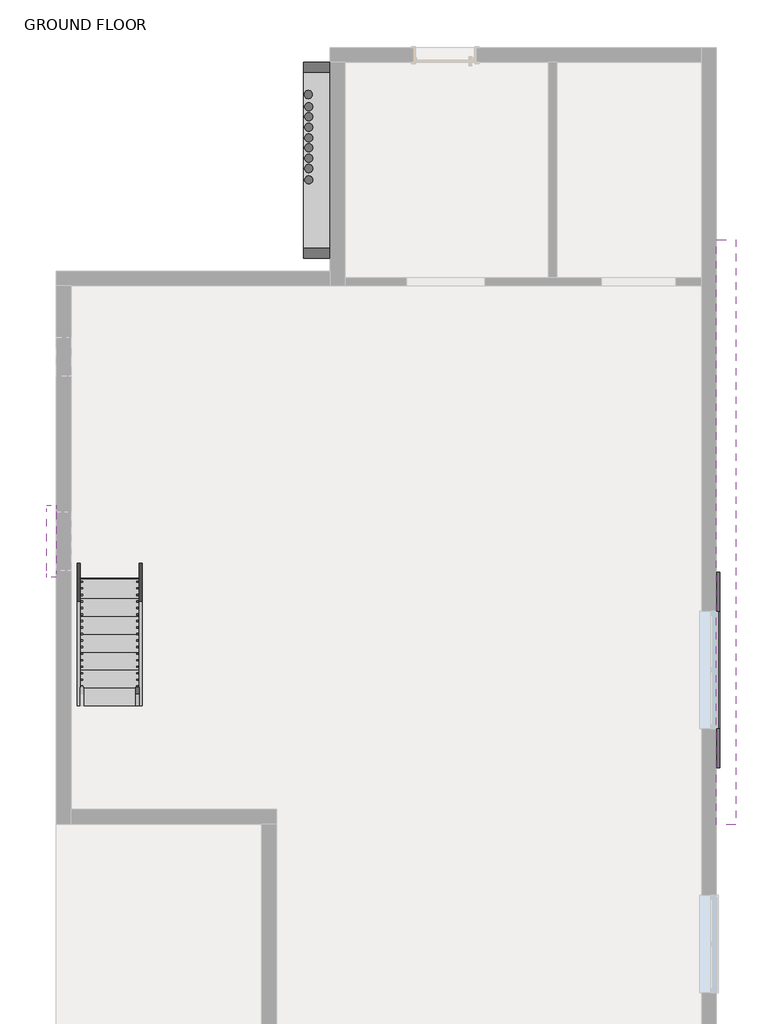
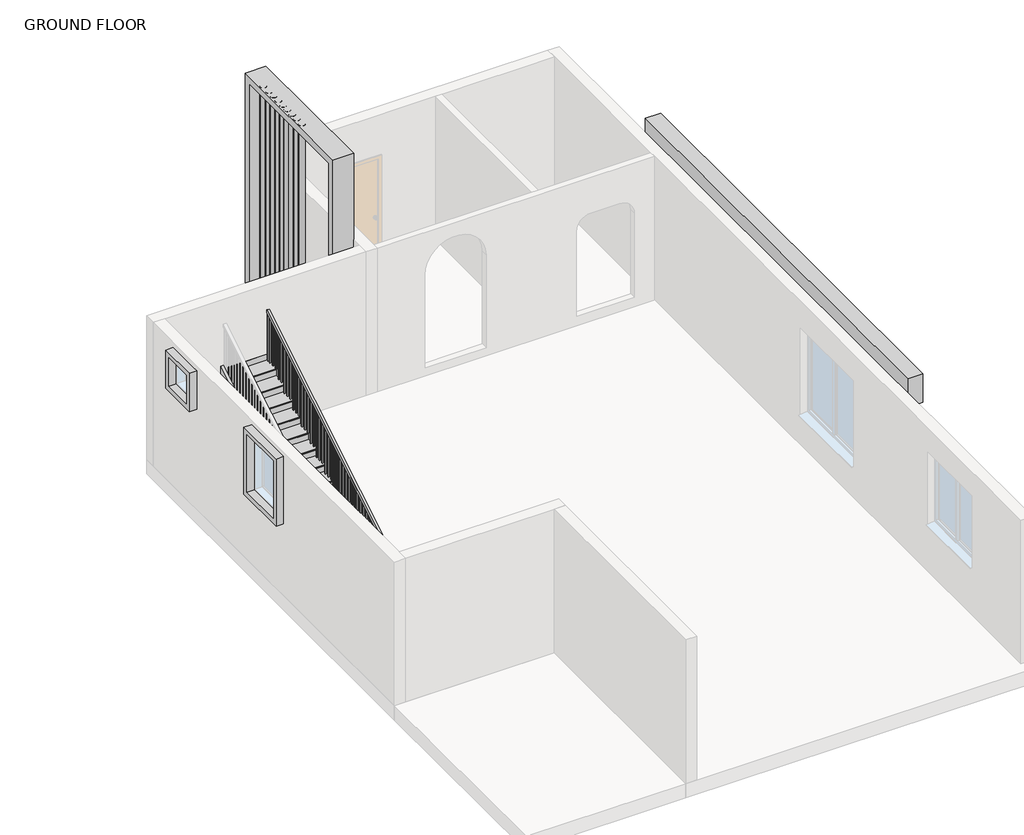
# One storey, part 2 of 2: 5 proxies, 2 members, 1 railing, 1 stair flight.
"""IFC4 building model written with IfcOpenShell, lengths in millimetres."""

from ifc_helpers import new_model, si_unit, frame, origin, place, context, project, spatial, polyline, outline, extrude, transform, mapped, element, save
from components import generic_models_1_generic_models_1_af82f8a7, generic_models_13_generic_models_13_70bfc34e, generic_models_16_generic_models_16_15e574d3, generic_models_17_generic_models_17_6d1cac68, generic_models_4_generic_models_4_9c707661, stair_flight_dba1ebb1

model = new_model("IFC4")

# Units and contexts
model_context = context("Model", 3, world=origin())
ifc_project = project(units=[si_unit("LENGTHUNIT", "METRE", prefix="MILLI")], contexts=[model_context])

# Site, building, storey
site = spatial("IfcSite", under=ifc_project)
building = spatial("IfcBuilding", under=site)
storey = spatial("IfcBuildingStorey", under=building, Name="GROUND FLOOR", Elevation=304.8)

# Proxies
placement = place(None, origin())
generic_models_1_generic_models_1_shape = generic_models_1_generic_models_1_af82f8a7(model_context)
element("IfcBuildingElementProxy", 1, Name="Generic Models 1 : Generic Models 1", ObjectType="Generic Models 1 : Generic Models 1", at=placement, inside=storey, context=model_context, shape_type="MappedRepresentation", body=[
    mapped(generic_models_1_generic_models_1_shape, transform((0.0, 0.0, 0.0), x_axis=(1.0, 0.0, 0.0), y_axis=(0.0, 1.0, 0.0), z_axis=(0.0, 0.0, 1.0))),
])
generic_models_13_generic_models_13_shape = generic_models_13_generic_models_13_70bfc34e(model_context)
element("IfcBuildingElementProxy", 2, Name="Generic Models 13 : Generic Models 13", ObjectType="Generic Models 13 : Generic Models 13", at=placement, inside=storey, context=model_context, shape_type="MappedRepresentation", body=[
    mapped(generic_models_13_generic_models_13_shape, transform((0.0, 0.0, 0.0), x_axis=(1.0, 0.0, 0.0), y_axis=(0.0, 1.0, 0.0), z_axis=(0.0, 0.0, 1.0))),
])
generic_models_16_generic_models_16_shape = generic_models_16_generic_models_16_15e574d3(model_context)
element("IfcBuildingElementProxy", 3, Name="Generic Models 16 : Generic Models 16", ObjectType="Generic Models 16 : Generic Models 16", at=placement, inside=storey, context=model_context, shape_type="MappedRepresentation", body=[
    mapped(generic_models_16_generic_models_16_shape, transform((0.0, 0.0, 0.0), x_axis=(1.0, 0.0, 0.0), y_axis=(0.0, 1.0, 0.0), z_axis=(0.0, 0.0, 1.0))),
])
generic_models_17_generic_models_17_shape = generic_models_17_generic_models_17_6d1cac68(model_context)
element("IfcBuildingElementProxy", 4, Name="Generic Models 17 : Generic Models 17", ObjectType="Generic Models 17 : Generic Models 17", at=placement, inside=storey, context=model_context, shape_type="MappedRepresentation", body=[
    mapped(generic_models_17_generic_models_17_shape, transform((0.0, 0.0, 0.0), x_axis=(1.0, 0.0, 0.0), y_axis=(0.0, 1.0, 0.0), z_axis=(0.0, 0.0, 1.0))),
])
generic_models_4_generic_models_4_shape = generic_models_4_generic_models_4_9c707661(model_context)
element("IfcBuildingElementProxy", 5, Name="Generic Models 4 : Generic Models 4", ObjectType="Generic Models 4 : Generic Models 4", at=placement, inside=storey, context=model_context, shape_type="MappedRepresentation", body=[
    mapped(generic_models_4_generic_models_4_shape, transform((0.0, 0.0, 0.0), x_axis=(1.0, 0.0, 0.0), y_axis=(0.0, 1.0, 0.0), z_axis=(0.0, 0.0, 1.0))),
])

# Members
element("IfcMember", 6, ObjectType="Stringer - 2\" Width", at=placement, inside=storey, context=model_context, shape_type="SweptSolid", body=[
    extrude(outline(polyline([(2020.7325341, 304.8), (2020.7325341, 516.914512), (6770.5325341, 3395.5811786), (6770.5325341, 3039.1724171), (2258.8180459, 304.8), (2020.7325341, 304.8)])), frame((-5772.3875748, 0.0, 0.0), z_axis=(1.0, 0.0, 0.0), x_axis=(0.0, 1.0, 0.0)), (0.0, 0.0, 1.0), 50.8),
])
element("IfcMember", 7, ObjectType="Stringer - 2\" Width", at=placement, inside=storey, context=model_context, shape_type="SweptSolid", body=[
    extrude(outline(polyline([(2020.7325341, 304.8), (2020.7325341, 516.914512), (6770.5325341, 3395.5811786), (6770.5325341, 3039.1724171), (2258.8180459, 304.8), (2020.7325341, 304.8)])), frame((-4807.1875748, 0.0, 0.0), z_axis=(1.0, 0.0, 0.0), x_axis=(0.0, 1.0, 0.0)), (0.0, 0.0, 1.0), 50.8),
])

# Railing
element("IfcRailing", 8, ObjectType="Handrail - Rectangular", at=placement, inside=storey, context=model_context, shape_type="SweptSolid", body=[
    extrude(outline(polyline([(2020.7325341, 1329.1318731), (2020.7325341, 1388.5333333), (6770.5325341, 4267.2), (6770.5325341, 4207.7985397), (2020.7325341, 1329.1318731)])), frame((-4857.9875748, 0.0, 0.0), z_axis=(1.0, 0.0, 0.0), x_axis=(0.0, 1.0, 0.0)), (0.0, 0.0, 1.0), 50.8),
    extrude(outline(polyline([(6684.8075341, 4155.8439943), (6703.8575341, 4167.3894488), (6703.8575341, 3183.4666667), (6684.8075341, 3183.4666667), (6684.8075341, 4155.8439943)])), frame((-4842.1125748, 0.0, 0.0), z_axis=(1.0, 0.0, 0.0), x_axis=(0.0, 1.0, 0.0)), (0.0, 0.0, 1.0), 19.05),
    extrude(outline(polyline([(6583.2075341, 4094.2682367), (6602.2575341, 4105.8136913), (6602.2575341, 3183.4666667), (6583.2075341, 3183.4666667), (6583.2075341, 4094.2682367)])), frame((-4842.1125748, 0.0, 0.0), z_axis=(1.0, 0.0, 0.0), x_axis=(0.0, 1.0, 0.0)), (0.0, 0.0, 1.0), 19.05),
    extrude(outline(polyline([(6481.6075341, 4032.6924791), (6500.6575341, 4044.2379337), (6500.6575341, 3183.4666667), (6481.6075341, 3183.4666667), (6481.6075341, 4032.6924791)])), frame((-4842.1125748, 0.0, 0.0), z_axis=(1.0, 0.0, 0.0), x_axis=(0.0, 1.0, 0.0)), (0.0, 0.0, 1.0), 19.05),
    extrude(outline(polyline([(6380.0075341, 3971.1167216), (6399.0575341, 3982.6621761), (6399.0575341, 3014.1333333), (6380.0075341, 3014.1333333), (6380.0075341, 3971.1167216)])), frame((-4842.1125748, 0.0, 0.0), z_axis=(1.0, 0.0, 0.0), x_axis=(0.0, 1.0, 0.0)), (0.0, 0.0, 1.0), 19.05),
    extrude(outline(polyline([(6278.4075341, 3909.540964), (6297.4575341, 3921.0864185), (6297.4575341, 3014.1333333), (6278.4075341, 3014.1333333), (6278.4075341, 3909.540964)])), frame((-4842.1125748, 0.0, 0.0), z_axis=(1.0, 0.0, 0.0), x_axis=(0.0, 1.0, 0.0)), (0.0, 0.0, 1.0), 19.05),
    extrude(outline(polyline([(6176.8075341, 3847.9652064), (6195.8575341, 3859.510661), (6195.8575341, 2844.8), (6176.8075341, 2844.8), (6176.8075341, 3847.9652064)])), frame((-4842.1125748, 0.0, 0.0), z_axis=(1.0, 0.0, 0.0), x_axis=(0.0, 1.0, 0.0)), (0.0, 0.0, 1.0), 19.05),
    extrude(outline(polyline([(6075.2075341, 3786.3894488), (6094.2575341, 3797.9349034), (6094.2575341, 2844.8), (6075.2075341, 2844.8), (6075.2075341, 3786.3894488)])), frame((-4842.1125748, 0.0, 0.0), z_axis=(1.0, 0.0, 0.0), x_axis=(0.0, 1.0, 0.0)), (0.0, 0.0, 1.0), 19.05),
    extrude(outline(polyline([(5973.6075341, 3724.8136913), (5992.6575341, 3736.3591458), (5992.6575341, 2844.8), (5973.6075341, 2844.8), (5973.6075341, 3724.8136913)])), frame((-4842.1125748, 0.0, 0.0), z_axis=(1.0, 0.0, 0.0), x_axis=(0.0, 1.0, 0.0)), (0.0, 0.0, 1.0), 19.05),
    extrude(outline(polyline([(5872.0075341, 3663.2379337), (5891.0575341, 3674.7833882), (5891.0575341, 2675.4666667), (5872.0075341, 2675.4666667), (5872.0075341, 3663.2379337)])), frame((-4842.1125748, 0.0, 0.0), z_axis=(1.0, 0.0, 0.0), x_axis=(0.0, 1.0, 0.0)), (0.0, 0.0, 1.0), 19.05),
    extrude(outline(polyline([(5770.4075341, 3601.6621761), (5789.4575341, 3613.2076307), (5789.4575341, 2675.4666667), (5770.4075341, 2675.4666667), (5770.4075341, 3601.6621761)])), frame((-4842.1125748, 0.0, 0.0), z_axis=(1.0, 0.0, 0.0), x_axis=(0.0, 1.0, 0.0)), (0.0, 0.0, 1.0), 19.05),
    extrude(outline(polyline([(5668.8075341, 3540.0864185), (5687.8575341, 3551.6318731), (5687.8575341, 2675.4666667), (5668.8075341, 2675.4666667), (5668.8075341, 3540.0864185)])), frame((-4842.1125748, 0.0, 0.0), z_axis=(1.0, 0.0, 0.0), x_axis=(0.0, 1.0, 0.0)), (0.0, 0.0, 1.0), 19.05),
    extrude(outline(polyline([(5567.2075341, 3478.510661), (5586.2575341, 3490.0561155), (5586.2575341, 2506.1333333), (5567.2075341, 2506.1333333), (5567.2075341, 3478.510661)])), frame((-4842.1125748, 0.0, 0.0), z_axis=(1.0, 0.0, 0.0), x_axis=(0.0, 1.0, 0.0)), (0.0, 0.0, 1.0), 19.05),
    extrude(outline(polyline([(5465.6075341, 3416.9349034), (5484.6575341, 3428.4803579), (5484.6575341, 2506.1333333), (5465.6075341, 2506.1333333), (5465.6075341, 3416.9349034)])), frame((-4842.1125748, 0.0, 0.0), z_axis=(1.0, 0.0, 0.0), x_axis=(0.0, 1.0, 0.0)), (0.0, 0.0, 1.0), 19.05),
    extrude(outline(polyline([(5364.0075341, 3355.3591458), (5383.0575341, 3366.9046004), (5383.0575341, 2506.1333333), (5364.0075341, 2506.1333333), (5364.0075341, 3355.3591458)])), frame((-4842.1125748, 0.0, 0.0), z_axis=(1.0, 0.0, 0.0), x_axis=(0.0, 1.0, 0.0)), (0.0, 0.0, 1.0), 19.05),
    extrude(outline(polyline([(5262.4075341, 3293.7833882), (5281.4575341, 3305.3288428), (5281.4575341, 2336.8), (5262.4075341, 2336.8), (5262.4075341, 3293.7833882)])), frame((-4842.1125748, 0.0, 0.0), z_axis=(1.0, 0.0, 0.0), x_axis=(0.0, 1.0, 0.0)), (0.0, 0.0, 1.0), 19.05),
    extrude(outline(polyline([(5160.8075341, 3232.2076307), (5179.8575341, 3243.7530852), (5179.8575341, 2336.8), (5160.8075341, 2336.8), (5160.8075341, 3232.2076307)])), frame((-4842.1125748, 0.0, 0.0), z_axis=(1.0, 0.0, 0.0), x_axis=(0.0, 1.0, 0.0)), (0.0, 0.0, 1.0), 19.05),
    extrude(outline(polyline([(5059.2075341, 3170.6318731), (5078.2575341, 3182.1773276), (5078.2575341, 2167.4666667), (5059.2075341, 2167.4666667), (5059.2075341, 3170.6318731)])), frame((-4842.1125748, 0.0, 0.0), z_axis=(1.0, 0.0, 0.0), x_axis=(0.0, 1.0, 0.0)), (0.0, 0.0, 1.0), 19.05),
    extrude(outline(polyline([(4957.6075341, 3109.0561155), (4976.6575341, 3120.60157), (4976.6575341, 2167.4666667), (4957.6075341, 2167.4666667), (4957.6075341, 3109.0561155)])), frame((-4842.1125748, 0.0, 0.0), z_axis=(1.0, 0.0, 0.0), x_axis=(0.0, 1.0, 0.0)), (0.0, 0.0, 1.0), 19.05),
    extrude(outline(polyline([(4856.0075341, 3047.4803579), (4875.0575341, 3059.0258125), (4875.0575341, 2167.4666667), (4856.0075341, 2167.4666667), (4856.0075341, 3047.4803579)])), frame((-4842.1125748, 0.0, 0.0), z_axis=(1.0, 0.0, 0.0), x_axis=(0.0, 1.0, 0.0)), (0.0, 0.0, 1.0), 19.05),
    extrude(outline(polyline([(4754.4075341, 2985.9046004), (4773.4575341, 2997.4500549), (4773.4575341, 1998.1333333), (4754.4075341, 1998.1333333), (4754.4075341, 2985.9046004)])), frame((-4842.1125748, 0.0, 0.0), z_axis=(1.0, 0.0, 0.0), x_axis=(0.0, 1.0, 0.0)), (0.0, 0.0, 1.0), 19.05),
    extrude(outline(polyline([(4652.8075341, 2924.3288428), (4671.8575341, 2935.8742973), (4671.8575341, 1998.1333333), (4652.8075341, 1998.1333333), (4652.8075341, 2924.3288428)])), frame((-4842.1125748, 0.0, 0.0), z_axis=(1.0, 0.0, 0.0), x_axis=(0.0, 1.0, 0.0)), (0.0, 0.0, 1.0), 19.05),
    extrude(outline(polyline([(4551.2075341, 2862.7530852), (4570.2575341, 2874.2985397), (4570.2575341, 1998.1333333), (4551.2075341, 1998.1333333), (4551.2075341, 2862.7530852)])), frame((-4842.1125748, 0.0, 0.0), z_axis=(1.0, 0.0, 0.0), x_axis=(0.0, 1.0, 0.0)), (0.0, 0.0, 1.0), 19.05),
    extrude(outline(polyline([(4449.6075341, 2801.1773276), (4468.6575341, 2812.7227822), (4468.6575341, 1828.8), (4449.6075341, 1828.8), (4449.6075341, 2801.1773276)])), frame((-4842.1125748, 0.0, 0.0), z_axis=(1.0, 0.0, 0.0), x_axis=(0.0, 1.0, 0.0)), (0.0, 0.0, 1.0), 19.05),
    extrude(outline(polyline([(4348.0075341, 2739.60157), (4367.0575341, 2751.1470246), (4367.0575341, 1828.8), (4348.0075341, 1828.8), (4348.0075341, 2739.60157)])), frame((-4842.1125748, 0.0, 0.0), z_axis=(1.0, 0.0, 0.0), x_axis=(0.0, 1.0, 0.0)), (0.0, 0.0, 1.0), 19.05),
    extrude(outline(polyline([(4246.4075341, 2678.0258125), (4265.4575341, 2689.571267), (4265.4575341, 1828.8), (4246.4075341, 1828.8), (4246.4075341, 2678.0258125)])), frame((-4842.1125748, 0.0, 0.0), z_axis=(1.0, 0.0, 0.0), x_axis=(0.0, 1.0, 0.0)), (0.0, 0.0, 1.0), 19.05),
    extrude(outline(polyline([(4144.8075341, 2616.4500549), (4163.8575341, 2627.9955094), (4163.8575341, 1659.4666667), (4144.8075341, 1659.4666667), (4144.8075341, 2616.4500549)])), frame((-4842.1125748, 0.0, 0.0), z_axis=(1.0, 0.0, 0.0), x_axis=(0.0, 1.0, 0.0)), (0.0, 0.0, 1.0), 19.05),
    extrude(outline(polyline([(4043.2075341, 2554.8742973), (4062.2575341, 2566.4197519), (4062.2575341, 1659.4666667), (4043.2075341, 1659.4666667), (4043.2075341, 2554.8742973)])), frame((-4842.1125748, 0.0, 0.0), z_axis=(1.0, 0.0, 0.0), x_axis=(0.0, 1.0, 0.0)), (0.0, 0.0, 1.0), 19.05),
    extrude(outline(polyline([(3941.6075341, 2493.2985397), (3960.6575341, 2504.8439943), (3960.6575341, 1490.1333333), (3941.6075341, 1490.1333333), (3941.6075341, 2493.2985397)])), frame((-4842.1125748, 0.0, 0.0), z_axis=(1.0, 0.0, 0.0), x_axis=(0.0, 1.0, 0.0)), (0.0, 0.0, 1.0), 19.05),
    extrude(outline(polyline([(3840.0075341, 2431.7227822), (3859.0575341, 2443.2682367), (3859.0575341, 1490.1333333), (3840.0075341, 1490.1333333), (3840.0075341, 2431.7227822)])), frame((-4842.1125748, 0.0, 0.0), z_axis=(1.0, 0.0, 0.0), x_axis=(0.0, 1.0, 0.0)), (0.0, 0.0, 1.0), 19.05),
    extrude(outline(polyline([(3738.4075341, 2370.1470246), (3757.4575341, 2381.6924791), (3757.4575341, 1490.1333333), (3738.4075341, 1490.1333333), (3738.4075341, 2370.1470246)])), frame((-4842.1125748, 0.0, 0.0), z_axis=(1.0, 0.0, 0.0), x_axis=(0.0, 1.0, 0.0)), (0.0, 0.0, 1.0), 19.05),
    extrude(outline(polyline([(3636.8075341, 2308.571267), (3655.8575341, 2320.1167216), (3655.8575341, 1320.8), (3636.8075341, 1320.8), (3636.8075341, 2308.571267)])), frame((-4842.1125748, 0.0, 0.0), z_axis=(1.0, 0.0, 0.0), x_axis=(0.0, 1.0, 0.0)), (0.0, 0.0, 1.0), 19.05),
    extrude(outline(polyline([(3535.2075341, 2246.9955094), (3554.2575341, 2258.540964), (3554.2575341, 1320.8), (3535.2075341, 1320.8), (3535.2075341, 2246.9955094)])), frame((-4842.1125748, 0.0, 0.0), z_axis=(1.0, 0.0, 0.0), x_axis=(0.0, 1.0, 0.0)), (0.0, 0.0, 1.0), 19.05),
    extrude(outline(polyline([(3433.6075341, 2185.4197519), (3452.6575341, 2196.9652064), (3452.6575341, 1320.8), (3433.6075341, 1320.8), (3433.6075341, 2185.4197519)])), frame((-4842.1125748, 0.0, 0.0), z_axis=(1.0, 0.0, 0.0), x_axis=(0.0, 1.0, 0.0)), (0.0, 0.0, 1.0), 19.05),
    extrude(outline(polyline([(3332.0075341, 2123.8439943), (3351.0575341, 2135.3894488), (3351.0575341, 1151.4666667), (3332.0075341, 1151.4666667), (3332.0075341, 2123.8439943)])), frame((-4842.1125748, 0.0, 0.0), z_axis=(1.0, 0.0, 0.0), x_axis=(0.0, 1.0, 0.0)), (0.0, 0.0, 1.0), 19.05),
    extrude(outline(polyline([(3230.4075341, 2062.2682367), (3249.4575341, 2073.8136913), (3249.4575341, 1151.4666667), (3230.4075341, 1151.4666667), (3230.4075341, 2062.2682367)])), frame((-4842.1125748, 0.0, 0.0), z_axis=(1.0, 0.0, 0.0), x_axis=(0.0, 1.0, 0.0)), (0.0, 0.0, 1.0), 19.05),
    extrude(outline(polyline([(3128.8075341, 2000.6924791), (3147.8575341, 2012.2379337), (3147.8575341, 1151.4666667), (3128.8075341, 1151.4666667), (3128.8075341, 2000.6924791)])), frame((-4842.1125748, 0.0, 0.0), z_axis=(1.0, 0.0, 0.0), x_axis=(0.0, 1.0, 0.0)), (0.0, 0.0, 1.0), 19.05),
    extrude(outline(polyline([(3027.2075341, 1939.1167216), (3046.2575341, 1950.6621761), (3046.2575341, 982.1333333), (3027.2075341, 982.1333333), (3027.2075341, 1939.1167216)])), frame((-4842.1125748, 0.0, 0.0), z_axis=(1.0, 0.0, 0.0), x_axis=(0.0, 1.0, 0.0)), (0.0, 0.0, 1.0), 19.05),
    extrude(outline(polyline([(2925.6075341, 1877.540964), (2944.6575341, 1889.0864185), (2944.6575341, 982.1333333), (2925.6075341, 982.1333333), (2925.6075341, 1877.540964)])), frame((-4842.1125748, 0.0, 0.0), z_axis=(1.0, 0.0, 0.0), x_axis=(0.0, 1.0, 0.0)), (0.0, 0.0, 1.0), 19.05),
    extrude(outline(polyline([(2824.0075341, 1815.9652064), (2843.0575341, 1827.510661), (2843.0575341, 812.8), (2824.0075341, 812.8), (2824.0075341, 1815.9652064)])), frame((-4842.1125748, 0.0, 0.0), z_axis=(1.0, 0.0, 0.0), x_axis=(0.0, 1.0, 0.0)), (0.0, 0.0, 1.0), 19.05),
    extrude(outline(polyline([(2722.4075341, 1754.3894488), (2741.4575341, 1765.9349034), (2741.4575341, 812.8), (2722.4075341, 812.8), (2722.4075341, 1754.3894488)])), frame((-4842.1125748, 0.0, 0.0), z_axis=(1.0, 0.0, 0.0), x_axis=(0.0, 1.0, 0.0)), (0.0, 0.0, 1.0), 19.05),
    extrude(outline(polyline([(2620.8075341, 1692.8136913), (2639.8575341, 1704.3591458), (2639.8575341, 812.8), (2620.8075341, 812.8), (2620.8075341, 1692.8136913)])), frame((-4842.1125748, 0.0, 0.0), z_axis=(1.0, 0.0, 0.0), x_axis=(0.0, 1.0, 0.0)), (0.0, 0.0, 1.0), 19.05),
    extrude(outline(polyline([(2519.2075341, 1631.2379337), (2538.2575341, 1642.7833882), (2538.2575341, 643.4666667), (2519.2075341, 643.4666667), (2519.2075341, 1631.2379337)])), frame((-4842.1125748, 0.0, 0.0), z_axis=(1.0, 0.0, 0.0), x_axis=(0.0, 1.0, 0.0)), (0.0, 0.0, 1.0), 19.05),
    extrude(outline(polyline([(2417.6075341, 1569.6621761), (2436.6575341, 1581.2076307), (2436.6575341, 643.4666667), (2417.6075341, 643.4666667), (2417.6075341, 1569.6621761)])), frame((-4842.1125748, 0.0, 0.0), z_axis=(1.0, 0.0, 0.0), x_axis=(0.0, 1.0, 0.0)), (0.0, 0.0, 1.0), 19.05),
    extrude(outline(polyline([(2316.0075341, 1508.0864185), (2335.0575341, 1519.6318731), (2335.0575341, 643.4666667), (2316.0075341, 643.4666667), (2316.0075341, 1508.0864185)])), frame((-4842.1125748, 0.0, 0.0), z_axis=(1.0, 0.0, 0.0), x_axis=(0.0, 1.0, 0.0)), (0.0, 0.0, 1.0), 19.05),
    extrude(outline(polyline([(2214.4075341, 1446.510661), (2233.4575341, 1458.0561155), (2233.4575341, 474.1333333), (2214.4075341, 474.1333333), (2214.4075341, 1446.510661)])), frame((-4842.1125748, 0.0, 0.0), z_axis=(1.0, 0.0, 0.0), x_axis=(0.0, 1.0, 0.0)), (0.0, 0.0, 1.0), 19.05),
    extrude(outline(polyline([(2112.8075341, 1384.9349034), (2131.8575341, 1396.4803579), (2131.8575341, 474.1333333), (2112.8075341, 474.1333333), (2112.8075341, 1384.9349034)])), frame((-4842.1125748, 0.0, 0.0), z_axis=(1.0, 0.0, 0.0), x_axis=(0.0, 1.0, 0.0)), (0.0, 0.0, 1.0), 19.05),
    extrude(outline(polyline([(6751.4825341, 4196.2530852), (6770.5325341, 4207.7985397), (6770.5325341, 3183.4666667), (6751.4825341, 3183.4666667), (6751.4825341, 4196.2530852)])), frame((-4842.1125748, 0.0, 0.0), z_axis=(1.0, 0.0, 0.0), x_axis=(0.0, 1.0, 0.0)), (0.0, 0.0, 1.0), 19.05),
    extrude(outline(polyline([(2020.7325341, 1329.1318731), (2039.7825341, 1340.6773276), (2039.7825341, 474.1333333), (2020.7325341, 474.1333333), (2020.7325341, 1329.1318731)])), frame((-4842.1125748, 0.0, 0.0), z_axis=(1.0, 0.0, 0.0), x_axis=(0.0, 1.0, 0.0)), (0.0, 0.0, 1.0), 19.05),
])

# Stair flight
stair_flight_shape = stair_flight_dba1ebb1(model_context)
element("IfcStairFlight", 9, ObjectType="2\" Tread 1\" Nosing 1/4\" Riser", at=placement, inside=storey, context=model_context, shape_type="MappedRepresentation", body=[
    mapped(stair_flight_shape, transform((0.0, 0.0, 0.0), x_axis=(1.0, 0.0, 0.0), y_axis=(0.0, 1.0, 0.0), z_axis=(0.0, 0.0, 1.0))),
])

save(model, "model.ifc")

# Revit data of these elements
# Type "Handrail - Rectangular"
#   Assembly Code = "C2010400"
#   built-in parameter 1008612 = 0.0416667 (stored number, unit not read)
#   built-in parameter 1008611 = 0.0416667 (stored number, unit not read)
#   built-in parameter 1008609 = 0.333333 (stored number, unit not read)
#   built-in parameter 1008604 = 0.166667 (stored number, unit not read)
#   built-in parameter 1008603 = 0.166667 (stored number, unit not read)
#   Railing Height = 3' - 0"
#   built-in parameter 1008630 = 2
#   built-in parameter 1008610 = 2
#   built-in parameter 1008618 = Baluster - Square : 3/4"
# Element 1 (IfcBuildingElementProxy, "Generic Models 1 : Generic Models 1")
#   Phase Created = New Construction
#   Materials on its faces: "OUTER WALL 9\""
# Element 2 (IfcBuildingElementProxy, "Generic Models 13 : Generic Models 13")
#   Phase Created = New Construction
#   Materials on its faces: "chocolate brown"
# Element 3 (IfcBuildingElementProxy, "Generic Models 16 : Generic Models 16")
#   Phase Created = New Construction
#   Materials on its faces: "chocolate brown"
# Element 4 (IfcBuildingElementProxy, "Generic Models 17 : Generic Models 17")
#   Phase Created = New Construction
#   Materials on its faces: "Cherry"
# Element 5 (IfcBuildingElementProxy, "Generic Models 4 : Generic Models 4")
#   Phase Created = New Construction
# Elements 6, 7 (IfcMember, "Stringer - 2\" Width")
#   Phase Created = New Construction
# Element 8 (IfcRailing, "Handrail - Rectangular")
#   Phase Created = New Construction
# Element 9 (IfcStairFlight, "2\" Tread 1\" Nosing 1/4\" Riser")
#   Phase Created = New Construction
# Materials
#   "OUTER WALL 9\"": class "Generic", colour RGB 120 120 120, transparency 0, Cost = 0
#   "chocolate brown": class "Generic", colour RGB 120 120 120, transparency 0, Cost = 0
#   "Cherry": class "Wood", colour RGB 226 177 128, transparency 0, Description = "Prunus Serotina", Cost = 0
